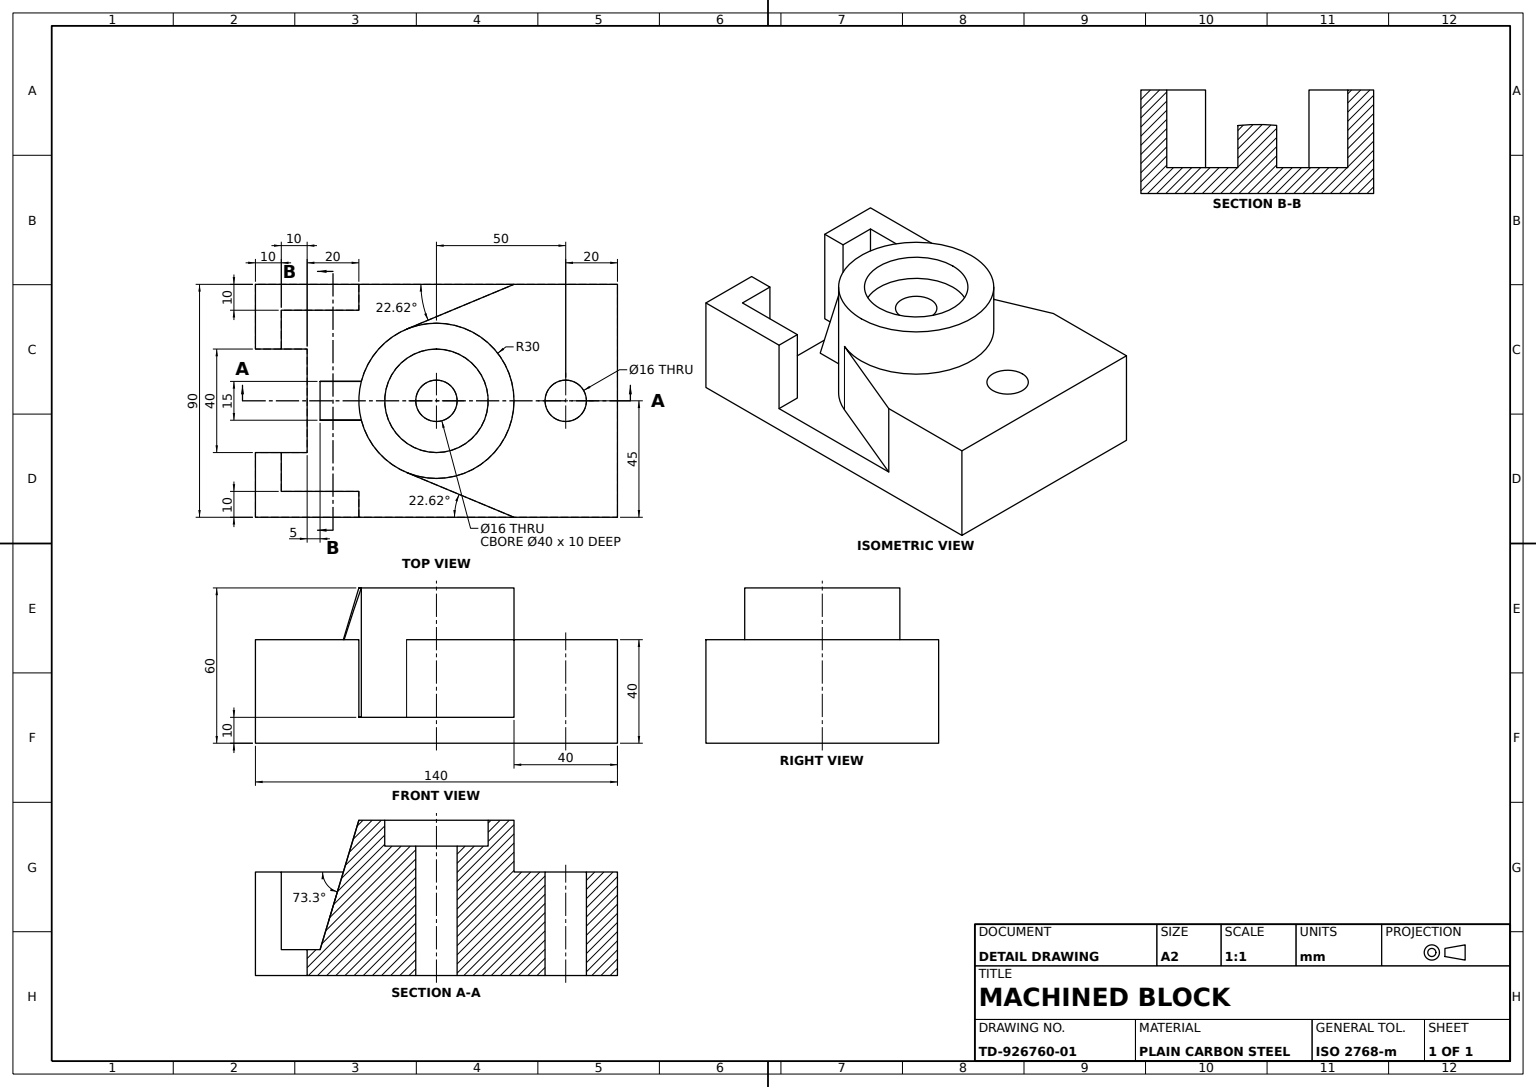
SolidWorks part; units mm, degrees
material "Plain Carbon Steel"
ref_plane "Front Plane" through (0, 0, 0) normal (0, 0, 1) x (1, 0, 0)
ref_plane "Top Plane" through (0, 0, 0) normal (0, 1, 0) x (1, 0, 0)
ref_plane "Right Plane" through (0, 0, 0) normal (1, 0, 0) x (0, 0, -1)
sketch "Base Plate Sketch" plane through (0, 0, 0) normal (0, 1, 0) x (1, 0, 0)
  line L1 (-70, -45) -> (70, -45)
  line L2 (-70, -45) -> (-70, 45)
  line L3 (-70, 45) -> (70, 45)
  line L4 (70, -45) -> (70, 45)
  line L5 (-70, -45) -> (70, 45) construction
  line L6 (-70, 45) -> (70, -45) construction
  point P0 (0, 0)
  dimension "D1" = 140
  dimension "D2" = 90
extrude "Base Plate" add sketch "Base Plate Sketch" along normal blind 40
sketch "Gland Boss Sketch" plane through (0, 0, 0) normal (0, 1, 0) x (1, 0, 0)
  circle A0 centre (0, 0) radius 20
  circle A1 centre (0, 0) radius 30
  dimension "D1" = 40
  dimension "D2" = 60
extrude "Gland Boss" add sketch "Gland Boss Sketch" along normal blind 60
sketch "Fork Cutout Sketch" plane through (0, 40, 0) normal (0, 1, 0) x (1, 0, 0)
  line L0 (-70, 20) -> (-60, 20)
  line L1 (-70, 45) -> (-70, -45) construction
  line L2 (-60, 20) -> (-60, 35)
  line L3 (-60, 35) -> (-30, 35)
  line L4 (-30, 35) -> (-30, 45)
  line L5 (70, 45) -> (-70, 45) construction
  line L8 (0, 0) -> (48.9365, 0) construction
  line L9 (-30, -35) -> (-30, -45)
  line L10 (-60, -35) -> (-30, -35)
  line L11 (-60, -20) -> (-60, -35)
  line L12 (-70, -20) -> (-60, -20)
  line L15 (-70, 20) -> (-70, -20)
  line L16 (-30, -45) -> (30, -45)
  line L17 (-70, -45) -> (70, -45) construction
  line L18 (-11.5385, -27.6923) -> (30, -45)
  line L19 (-30, 45) -> (30, 45)
  line L20 (-11.5385, 27.6923) -> (30, 45)
  circle A0 centre (0, 0) radius 30 construction
  circle A1 centre (0, 0) radius 30 construction
  arc A2 (-11.5385, 27.6923) -> (-11.5385, -27.6923) centre (0, 0) ccw
  dimension "D1" = 10
  dimension "D2" = 10
  dimension "D3" = 20
  dimension "D4" = 30
  dimension "D5" = 30
extrude "Fork Cutout" cut sketch "Fork Cutout Sketch" against normal blind 30
sketch "Bore and Hole Cut Sketch" plane through (0, 40, 0) normal (0, 1, 0) x (1, 0, 0)
  line L0 (70, -45) -> (70, 45) construction
  line L1 (-70, 20) -> (-70, -20) construction
  line L2 (-70, 20) -> (-50, 20)
  line L3 (-70, 20) -> (-70, -20)
  line L4 (-70, -20) -> (-50, -20)
  line L5 (-50, 20) -> (-50, -20)
  circle A0 centre (0, 0) radius 8
  circle A1 centre (50, 0) radius 8
  point P15 (-50, 0)
  dimension "D1" = 16
  dimension "D2" = 16
  dimension "D3" = 20
  dimension "D4" = 40
  dimension "D5" = 20
extrude "Bore and Hole Cut" cut sketch "Bore and Hole Cut Sketch" against normal up to next
sketch "Support Web Sketch" plane through (0, 60, 0) normal (0, 1, 0) x (1, 0, 0)
  line L0 (-50, 20) -> (-50, -20) construction
  line L1 (-29.0474, 7.5) -> (-45, 7.5)
  line L2 (-29.0474, 7.5) -> (-29.0474, -7.5)
  line L3 (-29.0474, -7.5) -> (-45, -7.5)
  line L4 (-45, 7.5) -> (-45, -7.5)
  circle A0 centre (0, 0) radius 30 construction
  dimension "D1" = 5
  dimension "D2" = 15
extrude "Support Web" add sketch "Support Web Sketch" against normal up to surface (50 mm away) up to face at (-31.5385, 10, 0)
sketch "Tapered Cut End Profile" plane through (0, 10, 0) normal (0, 1, 0) x (1, 0, 0)
  line L0 (-50, 20) -> (-50, -20) construction
  line L1 (-50, 15.4821) -> (-45, 15.4821)
  line L2 (-50, 15.4821) -> (-50, -14.5758)
  line L3 (-50, -14.5758) -> (-45, -14.5758)
  line L4 (-45, 15.4821) -> (-45, -14.5758)
  line L6 (-30, 35) -> (-60, 35) construction
  dimension "D1" = 5
  dimension "D2" = 19.5179
  dimension "D3" = 49.5758
sketch "Tapered Cut Start Profile" plane through (0, 60, 0) normal (0, 1, 0) x (1, 0, 0)
  line L1 (-29.0474, 7.5) -> (-45, 7.5)
  line L3 (-29.0474, -7.5) -> (-45, -7.5)
  line L4 (-45, 7.5) -> (-45, -7.5)
  arc A0 (-29.0474, 7.5) -> (-29.0474, -7.5) centre (0, 0) ccw
loft "Tapered Lofted Cut" cut profiles "Tapered Cut Start Profile", "Tapered Cut End Profile"
sketch "Lip Sketch" plane through (0, 40, 0) normal (0, 1, 0) x (1, 0, 0)
  circle A0 centre (0, 0) radius 8 construction
  circle A1 centre (0, 0) radius 20 construction
  circle A2 centre (0, 0) radius 8
  circle A3 centre (0, 0) radius 20
extrude "Lip 10mm" add sketch "Lip Sketch" along normal blind 10
